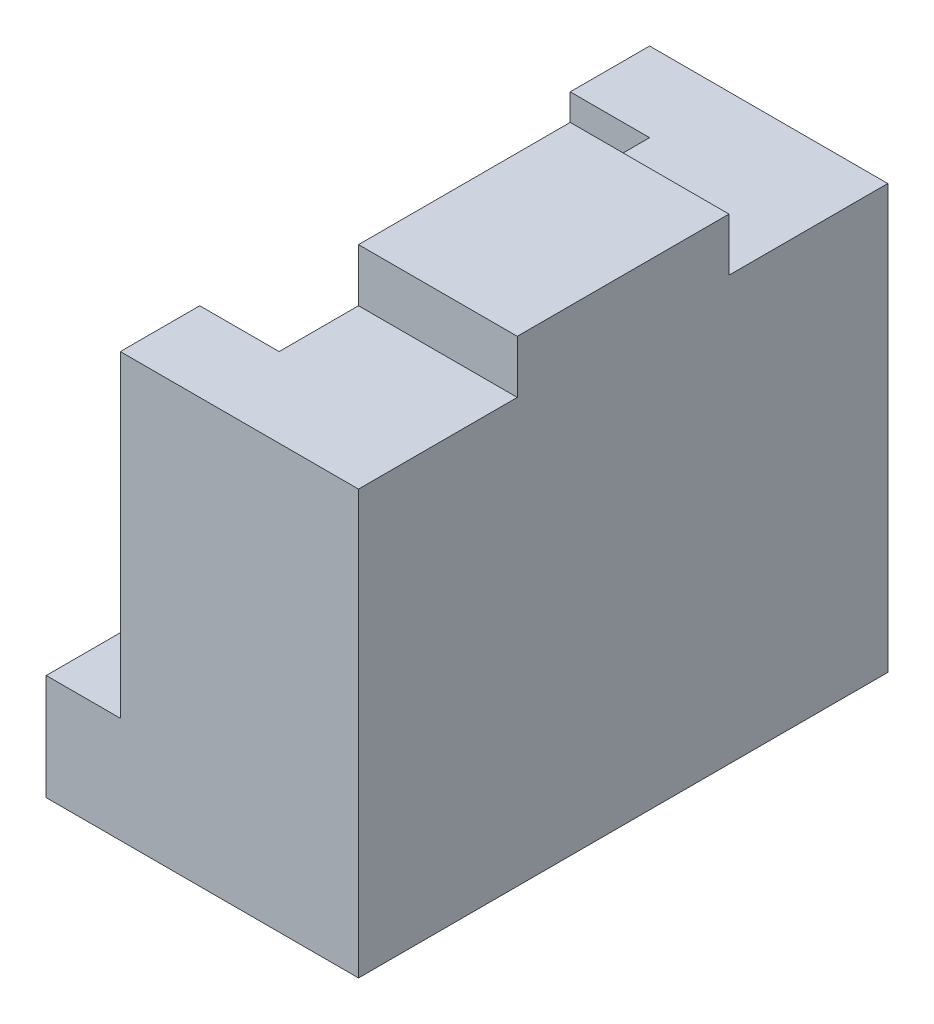
ISO-10303-21;
HEADER;
FILE_DESCRIPTION(('STEP AP214'),'2;1');
FILE_NAME('part.step','',(''),(''),'','','');
FILE_SCHEMA(('AUTOMOTIVE_DESIGN { 1 0 10303 214 1 1 1 1 }'));
ENDSEC;
DATA;
#1=APPLICATION_CONTEXT('core data for automotive mechanical design processes');
#2=APPLICATION_PROTOCOL_DEFINITION('international standard','automotive_design',2000,#1);
#3=PRODUCT_CONTEXT('',#1,'mechanical');
#4=PRODUCT('Part','Part','',(#3));
#5=PRODUCT_RELATED_PRODUCT_CATEGORY('part','',(#4));
#6=PRODUCT_DEFINITION_FORMATION('','',#4);
#7=PRODUCT_DEFINITION_CONTEXT('part definition',#1,'design');
#8=PRODUCT_DEFINITION('design','',#6,#7);
#9=PRODUCT_DEFINITION_SHAPE('','',#8);
#10=(LENGTH_UNIT() NAMED_UNIT(*) SI_UNIT(.MILLI.,.METRE.));
#11=(NAMED_UNIT(*) PLANE_ANGLE_UNIT() SI_UNIT($,.RADIAN.));
#12=(NAMED_UNIT(*) SI_UNIT($,.STERADIAN.) SOLID_ANGLE_UNIT());
#13=UNCERTAINTY_MEASURE_WITH_UNIT(LENGTH_MEASURE(1.E-05),#10,'distance_accuracy_value','');
#14=(GEOMETRIC_REPRESENTATION_CONTEXT(3) GLOBAL_UNCERTAINTY_ASSIGNED_CONTEXT((#13)) GLOBAL_UNIT_ASSIGNED_CONTEXT((#10,
#11,#12)) REPRESENTATION_CONTEXT('',''));
#15=CARTESIAN_POINT('',(0.,0.,0.));
#16=DIRECTION('',(0.,0.,1.));
#17=DIRECTION('',(1.,0.,0.));
#18=AXIS2_PLACEMENT_3D('',#15,#16,#17);
#19=CARTESIAN_POINT('',(-2112.11202744201,100.,250.));
#20=DIRECTION('',(0.,1.,0.));
#21=DIRECTION('',(0.,0.,1.));
#22=AXIS2_PLACEMENT_3D('',#19,#20,#21);
#23=PLANE('',#22);
#24=DIRECTION('',(1.,0.,0.));
#25=VECTOR('',#24,1.);
#26=CARTESIAN_POINT('',(-2112.11202744201,100.,250.));
#27=LINE('',#26,#25);
#28=CARTESIAN_POINT('',(50.,100.,250.));
#29=VERTEX_POINT('',#28);
#30=CARTESIAN_POINT('',(100.,100.,250.));
#31=VERTEX_POINT('',#30);
#32=EDGE_CURVE('E257',#29,#31,#27,.T.);
#33=ORIENTED_EDGE('',*,*,#32,.F.);
#34=DIRECTION('',(0.,0.,-1.));
#35=VECTOR('',#34,1.);
#36=CARTESIAN_POINT('',(50.,100.,750.));
#37=LINE('',#36,#35);
#38=CARTESIAN_POINT('',(49.9999999999998,100.,750.));
#39=VERTEX_POINT('',#38);
#40=EDGE_CURVE('E241',#39,#29,#37,.T.);
#41=ORIENTED_EDGE('',*,*,#40,.F.);
#42=DIRECTION('',(1.,0.,0.));
#43=VECTOR('',#42,1.);
#44=CARTESIAN_POINT('',(-2112.11202744201,100.,750.));
#45=LINE('',#44,#43);
#46=CARTESIAN_POINT('',(100.,100.,750.));
#47=VERTEX_POINT('',#46);
#48=EDGE_CURVE('E261',#39,#47,#45,.T.);
#49=ORIENTED_EDGE('',*,*,#48,.T.);
#50=DIRECTION('',(0.,0.,-1.));
#51=VECTOR('',#50,1.);
#52=CARTESIAN_POINT('',(100.,100.,250.));
#53=LINE('',#52,#51);
#54=EDGE_CURVE('E260',#47,#31,#53,.T.);
#55=ORIENTED_EDGE('',*,*,#54,.T.);
#56=EDGE_LOOP('',(#33,#41,#49,#55));
#57=FACE_BOUND('',#56,.T.);
#58=ADVANCED_FACE('F44',(#57),#23,.T.);
#59=CARTESIAN_POINT('',(540.,800.,1000.));
#60=DIRECTION('',(0.,-1.,0.));
#61=DIRECTION('',(0.,0.,-1.));
#62=AXIS2_PLACEMENT_3D('',#59,#60,#61);
#63=PLANE('',#62);
#64=DIRECTION('',(1.,0.,0.));
#65=VECTOR('',#64,1.);
#66=CARTESIAN_POINT('',(240.,800.,700.));
#67=LINE('',#66,#65);
#68=CARTESIAN_POINT('',(240.,800.,700.));
#69=VERTEX_POINT('',#68);
#70=CARTESIAN_POINT('',(540.,800.,700.));
#71=VERTEX_POINT('',#70);
#72=EDGE_CURVE('E290',#69,#71,#67,.T.);
#73=ORIENTED_EDGE('',*,*,#72,.F.);
#74=DIRECTION('',(0.,0.,-1.));
#75=VECTOR('',#74,1.);
#76=CARTESIAN_POINT('',(240.,800.,1000.));
#77=LINE('',#76,#75);
#78=CARTESIAN_POINT('',(240.,800.,850.));
#79=VERTEX_POINT('',#78);
#80=EDGE_CURVE('E361',#79,#69,#77,.T.);
#81=ORIENTED_EDGE('',*,*,#80,.F.);
#82=DIRECTION('',(-1.,0.,0.));
#83=VECTOR('',#82,1.);
#84=CARTESIAN_POINT('',(90.0000000000001,800.,850.));
#85=LINE('',#84,#83);
#86=CARTESIAN_POINT('',(90.0000000000001,800.,850.));
#87=VERTEX_POINT('',#86);
#88=EDGE_CURVE('E315',#79,#87,#85,.T.);
#89=ORIENTED_EDGE('',*,*,#88,.T.);
#90=DIRECTION('',(0.,0.,1.));
#91=VECTOR('',#90,1.);
#92=CARTESIAN_POINT('',(90.0000000000001,800.,850.));
#93=LINE('',#92,#91);
#94=CARTESIAN_POINT('',(90.0000000000001,800.,1000.));
#95=VERTEX_POINT('',#94);
#96=EDGE_CURVE('E321',#87,#95,#93,.T.);
#97=ORIENTED_EDGE('',*,*,#96,.T.);
#98=DIRECTION('',(-1.,0.,0.));
#99=VECTOR('',#98,1.);
#100=CARTESIAN_POINT('',(540.,800.,1000.));
#101=LINE('',#100,#99);
#102=CARTESIAN_POINT('',(540.,800.,1000.));
#103=VERTEX_POINT('',#102);
#104=EDGE_CURVE('E353',#103,#95,#101,.T.);
#105=ORIENTED_EDGE('',*,*,#104,.F.);
#106=DIRECTION('',(0.,0.,-1.));
#107=VECTOR('',#106,1.);
#108=CARTESIAN_POINT('',(540.,800.,1000.));
#109=LINE('',#108,#107);
#110=EDGE_CURVE('E52',#103,#71,#109,.T.);
#111=ORIENTED_EDGE('',*,*,#110,.T.);
#112=EDGE_LOOP('',(#73,#81,#89,#97,#105,#111));
#113=FACE_BOUND('',#112,.T.);
#114=ADVANCED_FACE('F401',(#113),#63,.F.);
#115=DIRECTION('',(-1.,0.,0.));
#116=VECTOR('',#115,1.);
#117=CARTESIAN_POINT('',(540.,800.,300.));
#118=LINE('',#117,#116);
#119=CARTESIAN_POINT('',(540.,800.,300.));
#120=VERTEX_POINT('',#119);
#121=CARTESIAN_POINT('',(240.,800.,300.));
#122=VERTEX_POINT('',#121);
#123=EDGE_CURVE('E278',#120,#122,#118,.T.);
#124=ORIENTED_EDGE('',*,*,#123,.F.);
#125=CARTESIAN_POINT('',(540.,800.,0.));
#126=VERTEX_POINT('',#125);
#127=EDGE_CURVE('E362',#120,#126,#109,.T.);
#128=ORIENTED_EDGE('',*,*,#127,.T.);
#129=DIRECTION('',(-1.,0.,0.));
#130=VECTOR('',#129,1.);
#131=CARTESIAN_POINT('',(540.,800.,0.));
#132=LINE('',#131,#130);
#133=CARTESIAN_POINT('',(90.0000000000001,800.,0.));
#134=VERTEX_POINT('',#133);
#135=EDGE_CURVE('E209',#126,#134,#132,.T.);
#136=ORIENTED_EDGE('',*,*,#135,.T.);
#137=DIRECTION('',(0.,0.,-1.));
#138=VECTOR('',#137,1.);
#139=CARTESIAN_POINT('',(90.0000000000001,800.,150.));
#140=LINE('',#139,#138);
#141=CARTESIAN_POINT('',(90.0000000000001,800.,150.));
#142=VERTEX_POINT('',#141);
#143=EDGE_CURVE('E341',#142,#134,#140,.T.);
#144=ORIENTED_EDGE('',*,*,#143,.F.);
#145=DIRECTION('',(1.,0.,0.));
#146=VECTOR('',#145,1.);
#147=CARTESIAN_POINT('',(240.,800.,150.));
#148=LINE('',#147,#146);
#149=CARTESIAN_POINT('',(240.,800.,150.));
#150=VERTEX_POINT('',#149);
#151=EDGE_CURVE('E338',#142,#150,#148,.T.);
#152=ORIENTED_EDGE('',*,*,#151,.T.);
#153=EDGE_CURVE('E365',#122,#150,#77,.T.);
#154=ORIENTED_EDGE('',*,*,#153,.F.);
#155=EDGE_LOOP('',(#124,#128,#136,#144,#152,#154));
#156=FACE_BOUND('',#155,.T.);
#157=ADVANCED_FACE('F371',(#156),#63,.F.);
#158=CARTESIAN_POINT('',(0.,0.,1000.));
#159=DIRECTION('',(0.,1.,0.));
#160=DIRECTION('',(0.,0.,1.));
#161=AXIS2_PLACEMENT_3D('',#158,#159,#160);
#162=PLANE('',#161);
#163=DIRECTION('',(1.,0.,0.));
#164=VECTOR('',#163,1.);
#165=CARTESIAN_POINT('',(0.,0.,0.));
#166=LINE('',#165,#164);
#167=CARTESIAN_POINT('',(-50.,0.,0.));
#168=VERTEX_POINT('',#167);
#169=CARTESIAN_POINT('',(540.,0.,0.));
#170=VERTEX_POINT('',#169);
#171=EDGE_CURVE('E213',#168,#170,#166,.T.);
#172=ORIENTED_EDGE('',*,*,#171,.T.);
#173=DIRECTION('',(0.,0.,-1.));
#174=VECTOR('',#173,1.);
#175=CARTESIAN_POINT('',(540.,0.,1000.));
#176=LINE('',#175,#174);
#177=CARTESIAN_POINT('',(540.,0.,1000.));
#178=VERTEX_POINT('',#177);
#179=EDGE_CURVE('E11',#178,#170,#176,.T.);
#180=ORIENTED_EDGE('',*,*,#179,.F.);
#181=DIRECTION('',(1.,0.,0.));
#182=VECTOR('',#181,1.);
#183=CARTESIAN_POINT('',(0.,0.,1000.));
#184=LINE('',#183,#182);
#185=CARTESIAN_POINT('',(-50.,0.,1000.));
#186=VERTEX_POINT('',#185);
#187=EDGE_CURVE('E206',#186,#178,#184,.T.);
#188=ORIENTED_EDGE('',*,*,#187,.F.);
#189=DIRECTION('',(0.,0.,1.));
#190=VECTOR('',#189,1.);
#191=CARTESIAN_POINT('',(-50.,0.,0.));
#192=LINE('',#191,#190);
#193=EDGE_CURVE('E216',#168,#186,#192,.T.);
#194=ORIENTED_EDGE('',*,*,#193,.F.);
#195=EDGE_LOOP('',(#172,#180,#188,#194));
#196=FACE_BOUND('',#195,.T.);
#197=ADVANCED_FACE('F50',(#196),#162,.F.);
#198=CARTESIAN_POINT('',(540.,0.,1000.));
#199=DIRECTION('',(-1.,0.,0.));
#200=DIRECTION('',(0.,0.,1.));
#201=AXIS2_PLACEMENT_3D('',#198,#199,#200);
#202=PLANE('',#201);
#203=DIRECTION('',(0.,1.,0.));
#204=VECTOR('',#203,1.);
#205=CARTESIAN_POINT('',(540.,0.,0.));
#206=LINE('',#205,#204);
#207=EDGE_CURVE('E357',#170,#126,#206,.T.);
#208=ORIENTED_EDGE('',*,*,#207,.T.);
#209=ORIENTED_EDGE('',*,*,#127,.F.);
#210=DIRECTION('',(0.,-1.,0.));
#211=VECTOR('',#210,1.);
#212=CARTESIAN_POINT('',(540.,900.,300.));
#213=LINE('',#212,#211);
#214=CARTESIAN_POINT('',(540.,900.,300.));
#215=VERTEX_POINT('',#214);
#216=EDGE_CURVE('E308',#215,#120,#213,.T.);
#217=ORIENTED_EDGE('',*,*,#216,.F.);
#218=DIRECTION('',(0.,0.,-1.));
#219=VECTOR('',#218,1.);
#220=CARTESIAN_POINT('',(540.,900.,700.));
#221=LINE('',#220,#219);
#222=CARTESIAN_POINT('',(540.,900.,700.));
#223=VERTEX_POINT('',#222);
#224=EDGE_CURVE('E288',#223,#215,#221,.T.);
#225=ORIENTED_EDGE('',*,*,#224,.F.);
#226=DIRECTION('',(0.,-1.,0.));
#227=VECTOR('',#226,1.);
#228=CARTESIAN_POINT('',(540.,900.,700.));
#229=LINE('',#228,#227);
#230=EDGE_CURVE('E294',#223,#71,#229,.T.);
#231=ORIENTED_EDGE('',*,*,#230,.T.);
#232=ORIENTED_EDGE('',*,*,#110,.F.);
#233=DIRECTION('',(0.,1.,0.));
#234=VECTOR('',#233,1.);
#235=CARTESIAN_POINT('',(540.,0.,1000.));
#236=LINE('',#235,#234);
#237=EDGE_CURVE('E346',#178,#103,#236,.T.);
#238=ORIENTED_EDGE('',*,*,#237,.F.);
#239=ORIENTED_EDGE('',*,*,#179,.T.);
#240=EDGE_LOOP('',(#208,#209,#217,#225,#231,#232,#238,#239));
#241=FACE_BOUND('',#240,.T.);
#242=ADVANCED_FACE('F374',(#241),#202,.F.);
#243=CARTESIAN_POINT('',(240.,800.,1000.));
#244=DIRECTION('',(1.,0.,0.));
#245=DIRECTION('',(0.,0.,-1.));
#246=AXIS2_PLACEMENT_3D('',#243,#244,#245);
#247=PLANE('',#246);
#248=DIRECTION('',(0.,0.,-1.));
#249=VECTOR('',#248,1.);
#250=CARTESIAN_POINT('',(240.,200.,1000.));
#251=LINE('',#250,#249);
#252=CARTESIAN_POINT('',(240.,200.,850.));
#253=VERTEX_POINT('',#252);
#254=CARTESIAN_POINT('',(240.,200.,150.));
#255=VERTEX_POINT('',#254);
#256=EDGE_CURVE('E351',#253,#255,#251,.T.);
#257=ORIENTED_EDGE('',*,*,#256,.F.);
#258=DIRECTION('',(0.,1.,0.));
#259=VECTOR('',#258,1.);
#260=CARTESIAN_POINT('',(240.,800.,850.));
#261=LINE('',#260,#259);
#262=EDGE_CURVE('E322',#253,#79,#261,.T.);
#263=ORIENTED_EDGE('',*,*,#262,.T.);
#264=ORIENTED_EDGE('',*,*,#80,.T.);
#265=DIRECTION('',(0.,-1.,0.));
#266=VECTOR('',#265,1.);
#267=CARTESIAN_POINT('',(240.,900.,700.));
#268=LINE('',#267,#266);
#269=CARTESIAN_POINT('',(240.,900.,700.));
#270=VERTEX_POINT('',#269);
#271=EDGE_CURVE('E305',#270,#69,#268,.T.);
#272=ORIENTED_EDGE('',*,*,#271,.F.);
#273=DIRECTION('',(0.,0.,1.));
#274=VECTOR('',#273,1.);
#275=CARTESIAN_POINT('',(240.,900.,300.));
#276=LINE('',#275,#274);
#277=CARTESIAN_POINT('',(240.,900.,300.));
#278=VERTEX_POINT('',#277);
#279=EDGE_CURVE('E293',#278,#270,#276,.T.);
#280=ORIENTED_EDGE('',*,*,#279,.F.);
#281=DIRECTION('',(0.,-1.,0.));
#282=VECTOR('',#281,1.);
#283=CARTESIAN_POINT('',(240.,900.,300.));
#284=LINE('',#283,#282);
#285=EDGE_CURVE('E304',#278,#122,#284,.T.);
#286=ORIENTED_EDGE('',*,*,#285,.T.);
#287=ORIENTED_EDGE('',*,*,#153,.T.);
#288=DIRECTION('',(0.,-1.,0.));
#289=VECTOR('',#288,1.);
#290=CARTESIAN_POINT('',(240.,200.,150.));
#291=LINE('',#290,#289);
#292=EDGE_CURVE('E334',#150,#255,#291,.T.);
#293=ORIENTED_EDGE('',*,*,#292,.T.);
#294=EDGE_LOOP('',(#257,#263,#264,#272,#280,#286,#287,#293));
#295=FACE_BOUND('',#294,.T.);
#296=ADVANCED_FACE('F389',(#295),#247,.F.);
#297=CARTESIAN_POINT('',(240.,200.,1000.));
#298=DIRECTION('',(0.,-1.,0.));
#299=DIRECTION('',(0.,0.,-1.));
#300=AXIS2_PLACEMENT_3D('',#297,#298,#299);
#301=PLANE('',#300);
#302=DIRECTION('',(0.,0.,-1.));
#303=VECTOR('',#302,1.);
#304=CARTESIAN_POINT('',(150.,200.,750.));
#305=LINE('',#304,#303);
#306=CARTESIAN_POINT('',(150.,200.,750.));
#307=VERTEX_POINT('',#306);
#308=CARTESIAN_POINT('',(150.,200.,250.));
#309=VERTEX_POINT('',#308);
#310=EDGE_CURVE('E268',#307,#309,#305,.T.);
#311=ORIENTED_EDGE('',*,*,#310,.F.);
#312=DIRECTION('',(-1.,0.,0.));
#313=VECTOR('',#312,1.);
#314=CARTESIAN_POINT('',(150.,200.,750.));
#315=LINE('',#314,#313);
#316=CARTESIAN_POINT('',(-50.,200.,750.));
#317=VERTEX_POINT('',#316);
#318=EDGE_CURVE('E279',#307,#317,#315,.T.);
#319=ORIENTED_EDGE('',*,*,#318,.T.);
#320=DIRECTION('',(0.,0.,-1.));
#321=VECTOR('',#320,1.);
#322=CARTESIAN_POINT('',(-50.,200.,1000.));
#323=LINE('',#322,#321);
#324=CARTESIAN_POINT('',(-50.,200.,1000.));
#325=VERTEX_POINT('',#324);
#326=EDGE_CURVE('E235',#325,#317,#323,.T.);
#327=ORIENTED_EDGE('',*,*,#326,.F.);
#328=DIRECTION('',(-1.,0.,0.));
#329=VECTOR('',#328,1.);
#330=CARTESIAN_POINT('',(240.,200.,1000.));
#331=LINE('',#330,#329);
#332=CARTESIAN_POINT('',(90.0000000000001,200.,1000.));
#333=VERTEX_POINT('',#332);
#334=EDGE_CURVE('E352',#333,#325,#331,.T.);
#335=ORIENTED_EDGE('',*,*,#334,.F.);
#336=DIRECTION('',(0.,0.,1.));
#337=VECTOR('',#336,1.);
#338=CARTESIAN_POINT('',(90.0000000000001,200.,850.));
#339=LINE('',#338,#337);
#340=CARTESIAN_POINT('',(90.0000000000001,200.,850.));
#341=VERTEX_POINT('',#340);
#342=EDGE_CURVE('E327',#341,#333,#339,.T.);
#343=ORIENTED_EDGE('',*,*,#342,.F.);
#344=DIRECTION('',(1.,0.,0.));
#345=VECTOR('',#344,1.);
#346=CARTESIAN_POINT('',(240.,200.,850.));
#347=LINE('',#346,#345);
#348=EDGE_CURVE('E319',#341,#253,#347,.T.);
#349=ORIENTED_EDGE('',*,*,#348,.T.);
#350=ORIENTED_EDGE('',*,*,#256,.T.);
#351=DIRECTION('',(-1.,0.,0.));
#352=VECTOR('',#351,1.);
#353=CARTESIAN_POINT('',(90.0000000000001,200.,150.));
#354=LINE('',#353,#352);
#355=CARTESIAN_POINT('',(90.0000000000001,200.,150.));
#356=VERTEX_POINT('',#355);
#357=EDGE_CURVE('E331',#255,#356,#354,.T.);
#358=ORIENTED_EDGE('',*,*,#357,.T.);
#359=DIRECTION('',(0.,0.,-1.));
#360=VECTOR('',#359,1.);
#361=CARTESIAN_POINT('',(90.0000000000001,200.,150.));
#362=LINE('',#361,#360);
#363=CARTESIAN_POINT('',(90.0000000000001,200.,0.));
#364=VERTEX_POINT('',#363);
#365=EDGE_CURVE('E205',#356,#364,#362,.T.);
#366=ORIENTED_EDGE('',*,*,#365,.T.);
#367=DIRECTION('',(-1.,0.,0.));
#368=VECTOR('',#367,1.);
#369=CARTESIAN_POINT('',(240.,200.,0.));
#370=LINE('',#369,#368);
#371=CARTESIAN_POINT('',(-50.,200.,0.));
#372=VERTEX_POINT('',#371);
#373=EDGE_CURVE('E197',#364,#372,#370,.T.);
#374=ORIENTED_EDGE('',*,*,#373,.T.);
#375=DIRECTION('',(0.,0.,-1.));
#376=VECTOR('',#375,1.);
#377=CARTESIAN_POINT('',(-50.,200.,250.));
#378=LINE('',#377,#376);
#379=CARTESIAN_POINT('',(-50.,200.,250.));
#380=VERTEX_POINT('',#379);
#381=EDGE_CURVE('E204',#380,#372,#378,.T.);
#382=ORIENTED_EDGE('',*,*,#381,.F.);
#383=DIRECTION('',(-1.,0.,0.));
#384=VECTOR('',#383,1.);
#385=CARTESIAN_POINT('',(150.,200.,250.));
#386=LINE('',#385,#384);
#387=EDGE_CURVE('E280',#309,#380,#386,.T.);
#388=ORIENTED_EDGE('',*,*,#387,.F.);
#389=EDGE_LOOP('',(#311,#319,#327,#335,#343,#349,#350,#358,#366,#374,#382,#388));
#390=FACE_BOUND('',#389,.T.);
#391=ADVANCED_FACE('F196',(#390),#301,.F.);
#392=CARTESIAN_POINT('',(0.,0.,1000.));
#393=DIRECTION('',(0.,0.,1.));
#394=DIRECTION('',(1.,0.,0.));
#395=AXIS2_PLACEMENT_3D('',#392,#393,#394);
#396=PLANE('',#395);
#397=ORIENTED_EDGE('',*,*,#334,.T.);
#398=DIRECTION('',(0.,1.,0.));
#399=VECTOR('',#398,1.);
#400=CARTESIAN_POINT('',(-50.,0.,1000.));
#401=LINE('',#400,#399);
#402=EDGE_CURVE('E230',#186,#325,#401,.T.);
#403=ORIENTED_EDGE('',*,*,#402,.F.);
#404=ORIENTED_EDGE('',*,*,#187,.T.);
#405=ORIENTED_EDGE('',*,*,#237,.T.);
#406=ORIENTED_EDGE('',*,*,#104,.T.);
#407=DIRECTION('',(0.,-1.,0.));
#408=VECTOR('',#407,1.);
#409=CARTESIAN_POINT('',(90.0000000000001,200.,1000.));
#410=LINE('',#409,#408);
#411=EDGE_CURVE('E311',#95,#333,#410,.T.);
#412=ORIENTED_EDGE('',*,*,#411,.T.);
#413=EDGE_LOOP('',(#397,#403,#404,#405,#406,#412));
#414=FACE_BOUND('',#413,.T.);
#415=ADVANCED_FACE('F411',(#414),#396,.T.);
#416=CARTESIAN_POINT('',(0.,0.,0.));
#417=DIRECTION('',(0.,0.,1.));
#418=DIRECTION('',(1.,0.,0.));
#419=AXIS2_PLACEMENT_3D('',#416,#417,#418);
#420=PLANE('',#419);
#421=ORIENTED_EDGE('',*,*,#171,.F.);
#422=DIRECTION('',(0.,-1.,0.));
#423=VECTOR('',#422,1.);
#424=CARTESIAN_POINT('',(-50.,200.,0.));
#425=LINE('',#424,#423);
#426=EDGE_CURVE('E215',#372,#168,#425,.T.);
#427=ORIENTED_EDGE('',*,*,#426,.F.);
#428=ORIENTED_EDGE('',*,*,#373,.F.);
#429=DIRECTION('',(0.,1.,0.));
#430=VECTOR('',#429,1.);
#431=CARTESIAN_POINT('',(90.0000000000001,800.,0.));
#432=LINE('',#431,#430);
#433=EDGE_CURVE('E326',#364,#134,#432,.T.);
#434=ORIENTED_EDGE('',*,*,#433,.T.);
#435=ORIENTED_EDGE('',*,*,#135,.F.);
#436=ORIENTED_EDGE('',*,*,#207,.F.);
#437=EDGE_LOOP('',(#421,#427,#428,#434,#435,#436));
#438=FACE_BOUND('',#437,.T.);
#439=ADVANCED_FACE('F214',(#438),#420,.F.);
#440=CARTESIAN_POINT('',(90.0000000000001,800.,150.));
#441=DIRECTION('',(-1.,0.,0.));
#442=DIRECTION('',(0.,0.,1.));
#443=AXIS2_PLACEMENT_3D('',#440,#441,#442);
#444=PLANE('',#443);
#445=ORIENTED_EDGE('',*,*,#433,.F.);
#446=ORIENTED_EDGE('',*,*,#365,.F.);
#447=DIRECTION('',(0.,1.,0.));
#448=VECTOR('',#447,1.);
#449=CARTESIAN_POINT('',(90.0000000000001,800.,150.));
#450=LINE('',#449,#448);
#451=EDGE_CURVE('E340',#356,#142,#450,.T.);
#452=ORIENTED_EDGE('',*,*,#451,.T.);
#453=ORIENTED_EDGE('',*,*,#143,.T.);
#454=EDGE_LOOP('',(#445,#446,#452,#453));
#455=FACE_BOUND('',#454,.T.);
#456=ADVANCED_FACE('F378',(#455),#444,.T.);
#457=CARTESIAN_POINT('',(0.,0.,150.));
#458=DIRECTION('',(0.,0.,1.));
#459=DIRECTION('',(1.,0.,0.));
#460=AXIS2_PLACEMENT_3D('',#457,#458,#459);
#461=PLANE('',#460);
#462=ORIENTED_EDGE('',*,*,#292,.F.);
#463=ORIENTED_EDGE('',*,*,#151,.F.);
#464=ORIENTED_EDGE('',*,*,#451,.F.);
#465=ORIENTED_EDGE('',*,*,#357,.F.);
#466=EDGE_LOOP('',(#462,#463,#464,#465));
#467=FACE_BOUND('',#466,.T.);
#468=ADVANCED_FACE('F381',(#467),#461,.T.);
#469=CARTESIAN_POINT('',(90.0000000000001,200.,850.));
#470=DIRECTION('',(-1.,0.,0.));
#471=DIRECTION('',(0.,0.,1.));
#472=AXIS2_PLACEMENT_3D('',#469,#470,#471);
#473=PLANE('',#472);
#474=ORIENTED_EDGE('',*,*,#411,.F.);
#475=ORIENTED_EDGE('',*,*,#96,.F.);
#476=DIRECTION('',(0.,-1.,0.));
#477=VECTOR('',#476,1.);
#478=CARTESIAN_POINT('',(90.0000000000001,200.,850.));
#479=LINE('',#478,#477);
#480=EDGE_CURVE('E314',#87,#341,#479,.T.);
#481=ORIENTED_EDGE('',*,*,#480,.T.);
#482=ORIENTED_EDGE('',*,*,#342,.T.);
#483=EDGE_LOOP('',(#474,#475,#481,#482));
#484=FACE_BOUND('',#483,.T.);
#485=ADVANCED_FACE('F414',(#484),#473,.T.);
#486=CARTESIAN_POINT('',(0.,0.,850.));
#487=DIRECTION('',(0.,0.,-1.));
#488=DIRECTION('',(-1.,0.,0.));
#489=AXIS2_PLACEMENT_3D('',#486,#487,#488);
#490=PLANE('',#489);
#491=ORIENTED_EDGE('',*,*,#88,.F.);
#492=ORIENTED_EDGE('',*,*,#262,.F.);
#493=ORIENTED_EDGE('',*,*,#348,.F.);
#494=ORIENTED_EDGE('',*,*,#480,.F.);
#495=EDGE_LOOP('',(#491,#492,#493,#494));
#496=FACE_BOUND('',#495,.T.);
#497=ADVANCED_FACE('F403',(#496),#490,.T.);
#498=CARTESIAN_POINT('',(540.,900.,300.));
#499=DIRECTION('',(0.,0.,1.));
#500=DIRECTION('',(1.,0.,0.));
#501=AXIS2_PLACEMENT_3D('',#498,#499,#500);
#502=PLANE('',#501);
#503=ORIENTED_EDGE('',*,*,#123,.T.);
#504=ORIENTED_EDGE('',*,*,#285,.F.);
#505=DIRECTION('',(-1.,0.,0.));
#506=VECTOR('',#505,1.);
#507=CARTESIAN_POINT('',(540.,900.,300.));
#508=LINE('',#507,#506);
#509=EDGE_CURVE('E287',#215,#278,#508,.T.);
#510=ORIENTED_EDGE('',*,*,#509,.F.);
#511=ORIENTED_EDGE('',*,*,#216,.T.);
#512=EDGE_LOOP('',(#503,#504,#510,#511));
#513=FACE_BOUND('',#512,.T.);
#514=ADVANCED_FACE('F391',(#513),#502,.F.);
#515=CARTESIAN_POINT('',(240.,900.,700.));
#516=DIRECTION('',(0.,0.,-1.));
#517=DIRECTION('',(-1.,0.,0.));
#518=AXIS2_PLACEMENT_3D('',#515,#516,#517);
#519=PLANE('',#518);
#520=ORIENTED_EDGE('',*,*,#72,.T.);
#521=ORIENTED_EDGE('',*,*,#230,.F.);
#522=DIRECTION('',(1.,0.,0.));
#523=VECTOR('',#522,1.);
#524=CARTESIAN_POINT('',(240.,900.,700.));
#525=LINE('',#524,#523);
#526=EDGE_CURVE('E291',#270,#223,#525,.T.);
#527=ORIENTED_EDGE('',*,*,#526,.F.);
#528=ORIENTED_EDGE('',*,*,#271,.T.);
#529=EDGE_LOOP('',(#520,#521,#527,#528));
#530=FACE_BOUND('',#529,.T.);
#531=ADVANCED_FACE('F402',(#530),#519,.F.);
#532=CARTESIAN_POINT('',(0.,900.,0.));
#533=DIRECTION('',(0.,1.,0.));
#534=DIRECTION('',(0.,0.,1.));
#535=AXIS2_PLACEMENT_3D('',#532,#533,#534);
#536=PLANE('',#535);
#537=ORIENTED_EDGE('',*,*,#224,.T.);
#538=ORIENTED_EDGE('',*,*,#509,.T.);
#539=ORIENTED_EDGE('',*,*,#279,.T.);
#540=ORIENTED_EDGE('',*,*,#526,.T.);
#541=EDGE_LOOP('',(#537,#538,#539,#540));
#542=FACE_BOUND('',#541,.T.);
#543=ADVANCED_FACE('F397',(#542),#536,.T.);
#544=CARTESIAN_POINT('',(150.,150.,750.));
#545=DIRECTION('',(0.,0.,1.));
#546=DIRECTION('',(1.,0.,0.));
#547=AXIS2_PLACEMENT_3D('',#544,#545,#546);
#548=PLANE('',#547);
#549=DIRECTION('',(-1.,0.,0.));
#550=VECTOR('',#549,1.);
#551=CARTESIAN_POINT('',(50.,50.0000000000001,750.));
#552=LINE('',#551,#550);
#553=CARTESIAN_POINT('',(50.,50.0000000000001,750.));
#554=VERTEX_POINT('',#553);
#555=CARTESIAN_POINT('',(-50.,50.0000000000001,750.));
#556=VERTEX_POINT('',#555);
#557=EDGE_CURVE('E249',#554,#556,#552,.T.);
#558=ORIENTED_EDGE('',*,*,#557,.T.);
#559=DIRECTION('',(0.,-1.,0.));
#560=VECTOR('',#559,1.);
#561=CARTESIAN_POINT('',(-50.,200.,750.));
#562=LINE('',#561,#560);
#563=EDGE_CURVE('E232',#317,#556,#562,.T.);
#564=ORIENTED_EDGE('',*,*,#563,.F.);
#565=ORIENTED_EDGE('',*,*,#318,.F.);
#566=DIRECTION('',(0.,1.,0.));
#567=VECTOR('',#566,1.);
#568=CARTESIAN_POINT('',(150.,150.,750.));
#569=LINE('',#568,#567);
#570=CARTESIAN_POINT('',(150.,150.,750.));
#571=VERTEX_POINT('',#570);
#572=EDGE_CURVE('E273',#571,#307,#569,.T.);
#573=ORIENTED_EDGE('',*,*,#572,.F.);
#574=DIRECTION('',(-1.,0.,0.));
#575=VECTOR('',#574,1.);
#576=CARTESIAN_POINT('',(150.,150.,750.));
#577=LINE('',#576,#575);
#578=CARTESIAN_POINT('',(100.,150.,750.));
#579=VERTEX_POINT('',#578);
#580=EDGE_CURVE('E282',#571,#579,#577,.T.);
#581=ORIENTED_EDGE('',*,*,#580,.T.);
#582=DIRECTION('',(0.,-1.,0.));
#583=VECTOR('',#582,1.);
#584=CARTESIAN_POINT('',(100.,100.,750.));
#585=LINE('',#584,#583);
#586=EDGE_CURVE('E254',#579,#47,#585,.T.);
#587=ORIENTED_EDGE('',*,*,#586,.T.);
#588=ORIENTED_EDGE('',*,*,#48,.F.);
#589=DIRECTION('',(0.,1.,0.));
#590=VECTOR('',#589,1.);
#591=CARTESIAN_POINT('',(50.,50.0000000000001,750.));
#592=LINE('',#591,#590);
#593=EDGE_CURVE('E58',#554,#39,#592,.T.);
#594=ORIENTED_EDGE('',*,*,#593,.F.);
#595=EDGE_LOOP('',(#558,#564,#565,#573,#581,#587,#588,#594));
#596=FACE_BOUND('',#595,.T.);
#597=ADVANCED_FACE('F423',(#596),#548,.F.);
#598=CARTESIAN_POINT('',(150.,150.,250.));
#599=DIRECTION('',(0.,-1.,0.));
#600=DIRECTION('',(0.,0.,-1.));
#601=AXIS2_PLACEMENT_3D('',#598,#599,#600);
#602=PLANE('',#601);
#603=DIRECTION('',(-1.,0.,0.));
#604=VECTOR('',#603,1.);
#605=CARTESIAN_POINT('',(150.,150.,250.));
#606=LINE('',#605,#604);
#607=CARTESIAN_POINT('',(150.,150.,250.));
#608=VERTEX_POINT('',#607);
#609=CARTESIAN_POINT('',(100.,150.,250.));
#610=VERTEX_POINT('',#609);
#611=EDGE_CURVE('E285',#608,#610,#606,.T.);
#612=ORIENTED_EDGE('',*,*,#611,.T.);
#613=DIRECTION('',(0.,0.,1.));
#614=VECTOR('',#613,1.);
#615=CARTESIAN_POINT('',(100.,150.,250.));
#616=LINE('',#615,#614);
#617=EDGE_CURVE('E70',#610,#579,#616,.T.);
#618=ORIENTED_EDGE('',*,*,#617,.T.);
#619=ORIENTED_EDGE('',*,*,#580,.F.);
#620=DIRECTION('',(0.,0.,1.));
#621=VECTOR('',#620,1.);
#622=CARTESIAN_POINT('',(150.,150.,250.));
#623=LINE('',#622,#621);
#624=EDGE_CURVE('E275',#608,#571,#623,.T.);
#625=ORIENTED_EDGE('',*,*,#624,.F.);
#626=EDGE_LOOP('',(#612,#618,#619,#625));
#627=FACE_BOUND('',#626,.T.);
#628=ADVANCED_FACE('F435',(#627),#602,.F.);
#629=CARTESIAN_POINT('',(150.,200.,250.));
#630=DIRECTION('',(0.,0.,-1.));
#631=DIRECTION('',(-1.,0.,0.));
#632=AXIS2_PLACEMENT_3D('',#629,#630,#631);
#633=PLANE('',#632);
#634=ORIENTED_EDGE('',*,*,#387,.T.);
#635=DIRECTION('',(0.,1.,0.));
#636=VECTOR('',#635,1.);
#637=CARTESIAN_POINT('',(-50.,50.0000000000001,250.));
#638=LINE('',#637,#636);
#639=CARTESIAN_POINT('',(-50.,50.0000000000001,250.));
#640=VERTEX_POINT('',#639);
#641=EDGE_CURVE('E221',#640,#380,#638,.T.);
#642=ORIENTED_EDGE('',*,*,#641,.F.);
#643=DIRECTION('',(-1.,0.,0.));
#644=VECTOR('',#643,1.);
#645=CARTESIAN_POINT('',(50.,50.0000000000001,250.));
#646=LINE('',#645,#644);
#647=CARTESIAN_POINT('',(50.,50.0000000000001,250.));
#648=VERTEX_POINT('',#647);
#649=EDGE_CURVE('E248',#648,#640,#646,.T.);
#650=ORIENTED_EDGE('',*,*,#649,.F.);
#651=DIRECTION('',(0.,-1.,0.));
#652=VECTOR('',#651,1.);
#653=CARTESIAN_POINT('',(50.,100.,250.));
#654=LINE('',#653,#652);
#655=EDGE_CURVE('E243',#29,#648,#654,.T.);
#656=ORIENTED_EDGE('',*,*,#655,.F.);
#657=ORIENTED_EDGE('',*,*,#32,.T.);
#658=DIRECTION('',(0.,1.,0.));
#659=VECTOR('',#658,1.);
#660=CARTESIAN_POINT('',(100.,150.,250.));
#661=LINE('',#660,#659);
#662=EDGE_CURVE('E259',#31,#610,#661,.T.);
#663=ORIENTED_EDGE('',*,*,#662,.T.);
#664=ORIENTED_EDGE('',*,*,#611,.F.);
#665=DIRECTION('',(0.,-1.,0.));
#666=VECTOR('',#665,1.);
#667=CARTESIAN_POINT('',(150.,200.,250.));
#668=LINE('',#667,#666);
#669=EDGE_CURVE('E270',#309,#608,#668,.T.);
#670=ORIENTED_EDGE('',*,*,#669,.F.);
#671=EDGE_LOOP('',(#634,#642,#650,#656,#657,#663,#664,#670));
#672=FACE_BOUND('',#671,.T.);
#673=ADVANCED_FACE('F430',(#672),#633,.F.);
#674=CARTESIAN_POINT('',(150.,0.,0.));
#675=DIRECTION('',(-1.,0.,0.));
#676=DIRECTION('',(0.,0.,1.));
#677=AXIS2_PLACEMENT_3D('',#674,#675,#676);
#678=PLANE('',#677);
#679=ORIENTED_EDGE('',*,*,#310,.T.);
#680=ORIENTED_EDGE('',*,*,#669,.T.);
#681=ORIENTED_EDGE('',*,*,#624,.T.);
#682=ORIENTED_EDGE('',*,*,#572,.T.);
#683=EDGE_LOOP('',(#679,#680,#681,#682));
#684=FACE_BOUND('',#683,.T.);
#685=ADVANCED_FACE('F431',(#684),#678,.T.);
#686=CARTESIAN_POINT('',(100.,200.,1000.));
#687=DIRECTION('',(1.,0.,0.));
#688=DIRECTION('',(0.,0.,-1.));
#689=AXIS2_PLACEMENT_3D('',#686,#687,#688);
#690=PLANE('',#689);
#691=ORIENTED_EDGE('',*,*,#617,.F.);
#692=ORIENTED_EDGE('',*,*,#662,.F.);
#693=ORIENTED_EDGE('',*,*,#54,.F.);
#694=ORIENTED_EDGE('',*,*,#586,.F.);
#695=EDGE_LOOP('',(#691,#692,#693,#694));
#696=FACE_BOUND('',#695,.T.);
#697=ADVANCED_FACE('F440',(#696),#690,.F.);
#698=CARTESIAN_POINT('',(50.,50.0000000000001,250.));
#699=DIRECTION('',(0.,-1.,0.));
#700=DIRECTION('',(0.,0.,-1.));
#701=AXIS2_PLACEMENT_3D('',#698,#699,#700);
#702=PLANE('',#701);
#703=ORIENTED_EDGE('',*,*,#649,.T.);
#704=DIRECTION('',(0.,0.,-1.));
#705=VECTOR('',#704,1.);
#706=CARTESIAN_POINT('',(-50.,50.0000000000001,750.));
#707=LINE('',#706,#705);
#708=EDGE_CURVE('E238',#556,#640,#707,.T.);
#709=ORIENTED_EDGE('',*,*,#708,.F.);
#710=ORIENTED_EDGE('',*,*,#557,.F.);
#711=DIRECTION('',(0.,0.,1.));
#712=VECTOR('',#711,1.);
#713=CARTESIAN_POINT('',(50.,50.0000000000001,250.));
#714=LINE('',#713,#712);
#715=EDGE_CURVE('E246',#648,#554,#714,.T.);
#716=ORIENTED_EDGE('',*,*,#715,.F.);
#717=EDGE_LOOP('',(#703,#709,#710,#716));
#718=FACE_BOUND('',#717,.T.);
#719=ADVANCED_FACE('F425',(#718),#702,.F.);
#720=CARTESIAN_POINT('',(50.,0.,0.));
#721=DIRECTION('',(-1.,0.,0.));
#722=DIRECTION('',(0.,0.,1.));
#723=AXIS2_PLACEMENT_3D('',#720,#721,#722);
#724=PLANE('',#723);
#725=ORIENTED_EDGE('',*,*,#40,.T.);
#726=ORIENTED_EDGE('',*,*,#655,.T.);
#727=ORIENTED_EDGE('',*,*,#715,.T.);
#728=ORIENTED_EDGE('',*,*,#593,.T.);
#729=EDGE_LOOP('',(#725,#726,#727,#728));
#730=FACE_BOUND('',#729,.T.);
#731=ADVANCED_FACE('F441',(#730),#724,.T.);
#732=CARTESIAN_POINT('',(-50.,0.,0.));
#733=DIRECTION('',(-1.,0.,0.));
#734=DIRECTION('',(0.,0.,1.));
#735=AXIS2_PLACEMENT_3D('',#732,#733,#734);
#736=PLANE('',#735);
#737=ORIENTED_EDGE('',*,*,#381,.T.);
#738=ORIENTED_EDGE('',*,*,#426,.T.);
#739=ORIENTED_EDGE('',*,*,#193,.T.);
#740=ORIENTED_EDGE('',*,*,#402,.T.);
#741=ORIENTED_EDGE('',*,*,#326,.T.);
#742=ORIENTED_EDGE('',*,*,#563,.T.);
#743=ORIENTED_EDGE('',*,*,#708,.T.);
#744=ORIENTED_EDGE('',*,*,#641,.T.);
#745=EDGE_LOOP('',(#737,#738,#739,#740,#741,#742,#743,#744));
#746=FACE_BOUND('',#745,.T.);
#747=ADVANCED_FACE('F224',(#746),#736,.T.);
#748=CLOSED_SHELL('',(#58,#114,#157,#197,#242,#296,#391,#415,#439,#456,#468,#485,#497,#514,#531,
#543,#597,#628,#673,#685,#697,#719,#731,#747));
#749=MANIFOLD_SOLID_BREP('B2',#748);
#750=ADVANCED_BREP_SHAPE_REPRESENTATION('',(#18,#749),#14);
#751=SHAPE_DEFINITION_REPRESENTATION(#9,#750);
ENDSEC;
END-ISO-10303-21;
